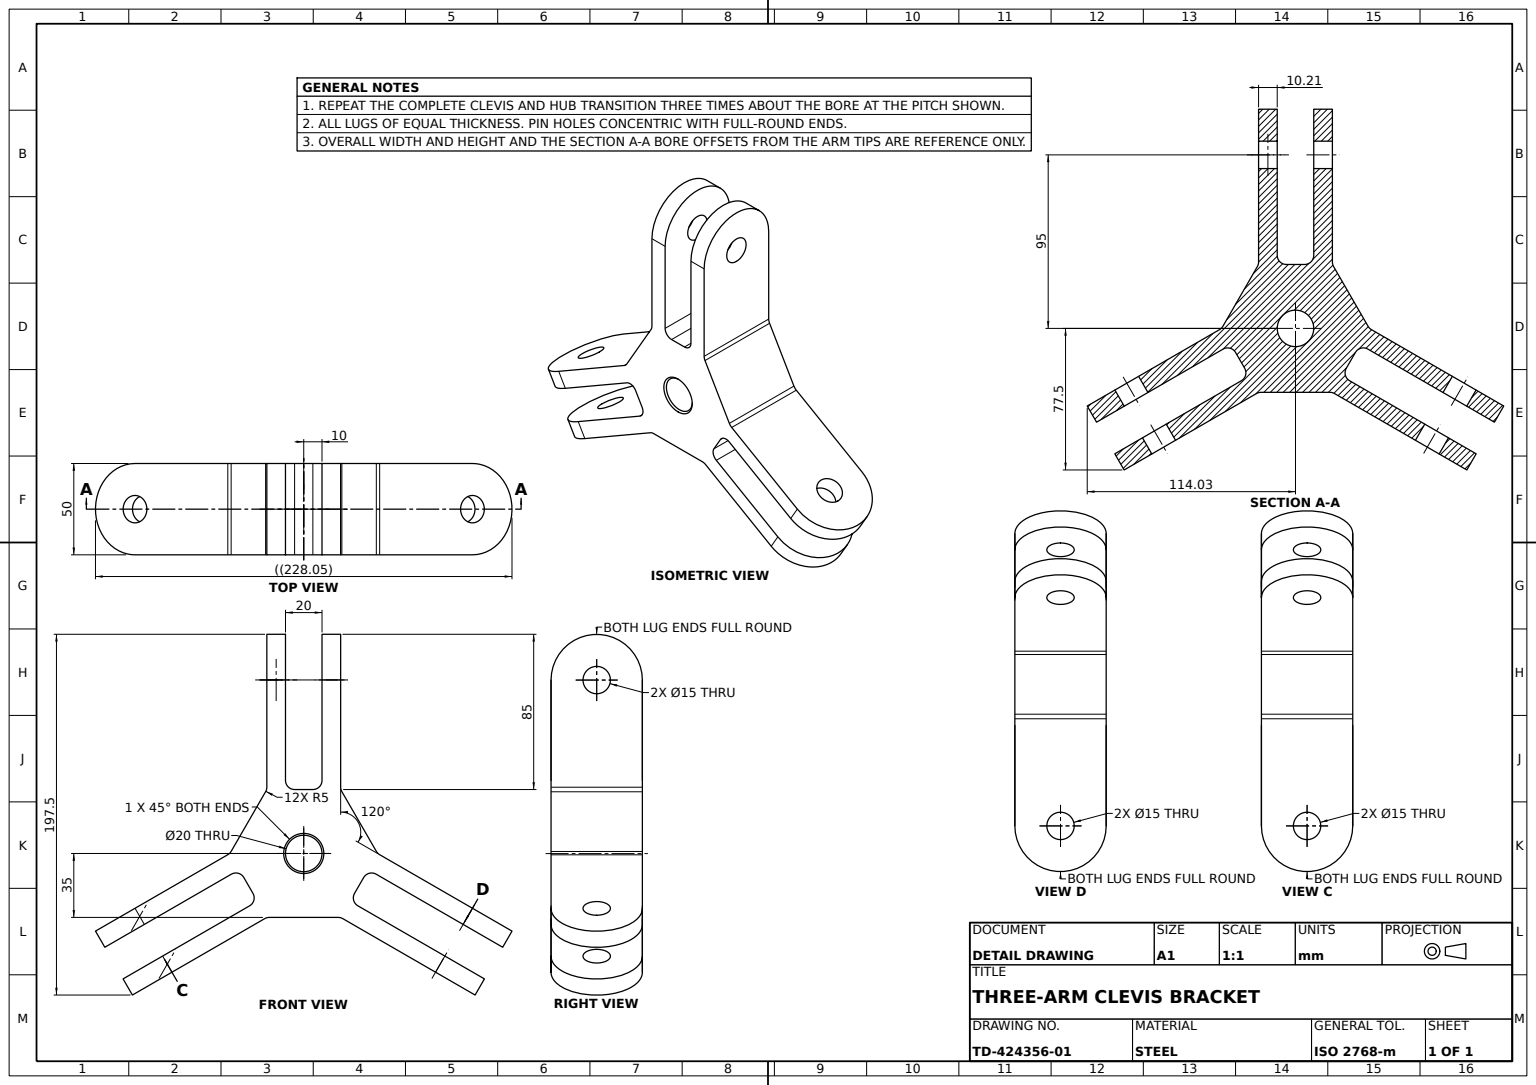
from build123d import *

# Parameters (mm, degrees)
THREE_ARM_BODY_50MM_DEPTH = 25
ARM_END_ROUND_B_RADIUS    = 25
ARM_END_ROUND_B_LENGTH    = 10.207259422
ARM_EDGE_FILLET_1_RADIUS  = 25
ARM_EDGE_FILLET_1_LENGTH  = 10.207259422
ARM_END_ROUND_A_RADIUS    = 25
ARM_END_ROUND_A_LENGTH    = 10.207259422
ARM_EDGE_FILLET_2_RADIUS  = 25
ARM_EDGE_FILLET_2_LENGTH  = 10.207259422
ARM_EDGE_FILLET_3_RADIUS  = 25
ARM_EDGE_FILLET_3_LENGTH  = 10.207259422
ARM_END_ROUND_C_RADIUS    = 25
ARM_END_ROUND_C_LENGTH    = 10.207259422
PIN_HOLE_A_15_REACH       = 188.921
PIN_HOLE_A_SKETCH_R       = 7.5
PIN_HOLE_B_15_REACH       = 188.921
PIN_HOLE_B_SKETCH_R       = 7.5
PIN_HOLE_C_15_REACH       = 183.779
PIN_HOLE_C_SKETCH_R       = 7.5
CENTER_BORE_SKETCH_R      = 10
CENTER_BORE_20_DEPTH      = 50
HUB_FILLET_R5_1_R         = 5
HUB_FILLET_R5_2_R         = 5
BORE_CHAMFER_1X45_SIZE    = 1


with BuildPart() as part:
    # Three-Arm Profile Sketch → Three-Arm Body 50mm (new, symmetric)
    with BuildSketch(Plane(origin=(0, 0, 0), x_dir=(1, 0, 0), z_dir=(0, 1, 0))):
        Polygon((-20.207259422, 35), (-20.207259422, 120), (-10, 120), (-10, 35), (10, 35), (10, 120), (20.207259422, 120), (20.207259422, 35), (40.414518843, 0), (114.026678165, -42.5), (108.923048454, -51.339745962), (35.310889132, -8.839745962), (25.310889132, -26.160254038), (98.923048454, -68.660254038), (93.819418743, -77.5), (20.207259422, -35), (-20.207259422, -35), (-93.819418743, -77.5), (-98.923048454, -68.660254038), (-25.310889132, -26.160254038), (-35.310889132, -8.839745962), (-108.923048454, -51.339745962), (-114.026678165, -42.5), (-40.414518843, 0), align=None)
    extrude(amount=THREE_ARM_BODY_50MM_DEPTH, both=True)

    # Arm End Round B: full round fillet: the end face becomes a half cylinder, R = half its width
    arm_end_round_b_face = Plane((-96.371233599, 0, 73.080127019), x_dir=(0.5, 0, 0.866025403784), z_dir=(-0.866025403784, 0, 0.5))  # on the end face: x along it, z out of the body
    arm_end_round_b_slab = arm_end_round_b_face.offset(-ARM_END_ROUND_B_RADIUS / 2) * Box(ARM_END_ROUND_B_LENGTH, 2 * ARM_END_ROUND_B_RADIUS, ARM_END_ROUND_B_RADIUS, mode=Mode.PRIVATE)  # the body's end, R deep
    arm_end_round_b_round = Plane((-74.720598504, 0, 60.580127019), x_dir=(-0.866025403784, 0, 0.5), z_dir=(0.5, 0, 0.866025403784)) * Cylinder(ARM_END_ROUND_B_RADIUS, ARM_END_ROUND_B_LENGTH, mode=Mode.PRIVATE)  # its axis R under the face
    add(arm_end_round_b_slab - arm_end_round_b_round, mode=Mode.SUBTRACT)

    # Arm Edge Fillet 1: full round fillet: the end face becomes a half cylinder, R = half its width
    arm_edge_fillet_1_face = Plane((-111.47486331, 0, 46.919872981), x_dir=(0.5, 0, 0.866025403784), z_dir=(-0.866025403784, 0, 0.5))  # on the end face: x along it, z out of the body
    arm_edge_fillet_1_slab = arm_edge_fillet_1_face.offset(-ARM_EDGE_FILLET_1_RADIUS / 2) * Box(ARM_EDGE_FILLET_1_LENGTH, 2 * ARM_EDGE_FILLET_1_RADIUS, ARM_EDGE_FILLET_1_RADIUS, mode=Mode.PRIVATE)  # the body's end, R deep
    arm_edge_fillet_1_round = Plane((-89.824228215, 0, 34.419872981), x_dir=(-0.866025403784, 0, 0.5), z_dir=(0.5, 0, 0.866025403784)) * Cylinder(ARM_EDGE_FILLET_1_RADIUS, ARM_EDGE_FILLET_1_LENGTH, mode=Mode.PRIVATE)  # its axis R under the face
    add(arm_edge_fillet_1_slab - arm_edge_fillet_1_round, mode=Mode.SUBTRACT)

    # Arm End Round A: full round fillet: the end face becomes a half cylinder, R = half its width
    arm_end_round_a_face = Plane((96.371233599, 0, 73.080127019), x_dir=(0.5, 0, -0.866025403784), z_dir=(0.866025403784, 0, 0.5))  # on the end face: x along it, z out of the body
    arm_end_round_a_slab = arm_end_round_a_face.offset(-ARM_END_ROUND_A_RADIUS / 2) * Box(ARM_END_ROUND_A_LENGTH, 2 * ARM_END_ROUND_A_RADIUS, ARM_END_ROUND_A_RADIUS, mode=Mode.PRIVATE)  # the body's end, R deep
    arm_end_round_a_round = Plane((74.720598504, 0, 60.580127019), x_dir=(0.866025403784, 0, 0.5), z_dir=(0.5, 0, -0.866025403784)) * Cylinder(ARM_END_ROUND_A_RADIUS, ARM_END_ROUND_A_LENGTH, mode=Mode.PRIVATE)  # its axis R under the face
    add(arm_end_round_a_slab - arm_end_round_a_round, mode=Mode.SUBTRACT)

    # Arm Edge Fillet 2: full round fillet: the end face becomes a half cylinder, R = half its width
    arm_edge_fillet_2_face = Plane((111.47486331, 0, 46.919872981), x_dir=(0.5, 0, -0.866025403784), z_dir=(0.866025403784, 0, 0.5))  # on the end face: x along it, z out of the body
    arm_edge_fillet_2_slab = arm_edge_fillet_2_face.offset(-ARM_EDGE_FILLET_2_RADIUS / 2) * Box(ARM_EDGE_FILLET_2_LENGTH, 2 * ARM_EDGE_FILLET_2_RADIUS, ARM_EDGE_FILLET_2_RADIUS, mode=Mode.PRIVATE)  # the body's end, R deep
    arm_edge_fillet_2_round = Plane((89.824228215, 0, 34.419872981), x_dir=(0.866025403784, 0, 0.5), z_dir=(0.5, 0, -0.866025403784)) * Cylinder(ARM_EDGE_FILLET_2_RADIUS, ARM_EDGE_FILLET_2_LENGTH, mode=Mode.PRIVATE)  # its axis R under the face
    add(arm_edge_fillet_2_slab - arm_edge_fillet_2_round, mode=Mode.SUBTRACT)

    # Arm Edge Fillet 3: full round fillet: the end face becomes a half cylinder, R = half its width
    arm_edge_fillet_3_face = Plane((15.103629711, 0, -120), x_dir=(-1, 0, 0), z_dir=(0, 0, -1))  # on the end face: x along it, z out of the body
    arm_edge_fillet_3_slab = arm_edge_fillet_3_face.offset(-ARM_EDGE_FILLET_3_RADIUS / 2) * Box(ARM_EDGE_FILLET_3_LENGTH, 2 * ARM_EDGE_FILLET_3_RADIUS, ARM_EDGE_FILLET_3_RADIUS, mode=Mode.PRIVATE)  # the body's end, R deep
    arm_edge_fillet_3_round = Plane((15.103629711, 0, -95), x_dir=(0, 0, -1), z_dir=(-1, 0, 0)) * Cylinder(ARM_EDGE_FILLET_3_RADIUS, ARM_EDGE_FILLET_3_LENGTH, mode=Mode.PRIVATE)  # its axis R under the face
    add(arm_edge_fillet_3_slab - arm_edge_fillet_3_round, mode=Mode.SUBTRACT)

    # Arm End Round C: full round fillet: the end face becomes a half cylinder, R = half its width
    arm_end_round_c_face = Plane((-15.103629711, 0, -120), x_dir=(1, 0, 0), z_dir=(0, 0, -1))  # on the end face: x along it, z out of the body
    arm_end_round_c_slab = arm_end_round_c_face.offset(-ARM_END_ROUND_C_RADIUS / 2) * Box(ARM_END_ROUND_C_LENGTH, 2 * ARM_END_ROUND_C_RADIUS, ARM_END_ROUND_C_RADIUS, mode=Mode.PRIVATE)  # the body's end, R deep
    arm_end_round_c_round = Plane((-15.103629711, 0, -95), x_dir=(0, 0, -1), z_dir=(1, 0, 0)) * Cylinder(ARM_END_ROUND_C_RADIUS, ARM_END_ROUND_C_LENGTH, mode=Mode.PRIVATE)  # its axis R under the face
    add(arm_end_round_c_slab - arm_end_round_c_round, mode=Mode.SUBTRACT)

    # Pin Hole A _15: up to this face of the body (flat: up to its plane)
    pin_hole_a_15_end = Plane(part.part.faces().sort_by_distance((75.066762447, 0, 20.006482173))[0])
    # Pin Hole A Sketch → Pin Hole A _15 (cut, up to the picked face)
    with BuildSketch(Plane(origin=(-10.103629711, 0, 17.5), x_dir=(0.8660254037844392, 0, 0.49999999999999917), z_dir=(-0.49999999999999917, 0, 0.8660254037844392)), mode=Mode.PRIVATE) as pin_hole_a_15_sk1:
        with Locations((95, 0)):
            Circle(PIN_HOLE_A_SKETCH_R)
    pin_hole_a_15_tool1 = split(extrude(pin_hole_a_15_sk1.sketch, amount=-PIN_HOLE_A_15_REACH, mode=Mode.PRIVATE), bisect_by=pin_hole_a_15_end, keep=Keep.BOTH, mode=Mode.PRIVATE)
    add(pin_hole_a_15_tool1.solids().sort_by(Axis((72.168784, 0, 65), (0.49999999999999917, 0, -0.8660254037844392)))[0], mode=Mode.SUBTRACT)

    # Pin Hole B _15: up to this face of the body (flat: up to its plane)
    pin_hole_b_15_end = Plane(part.part.faces().sort_by_distance((-75.066762447, 0, 20.006482173))[0])
    # Pin Hole B Sketch → Pin Hole B _15 (cut, up to the picked face)
    with BuildSketch(Plane(origin=(10.103629711, 0, 17.5), x_dir=(0.86602540378444, 0, -0.4999999999999976), z_dir=(0.4999999999999976, 0, 0.86602540378444)), mode=Mode.PRIVATE) as pin_hole_b_15_sk1:
        with Locations((-95, 0)):
            Circle(PIN_HOLE_B_SKETCH_R)
    pin_hole_b_15_tool1 = split(extrude(pin_hole_b_15_sk1.sketch, amount=-PIN_HOLE_B_15_REACH, mode=Mode.PRIVATE), bisect_by=pin_hole_b_15_end, keep=Keep.BOTH, mode=Mode.PRIVATE)
    add(pin_hole_b_15_tool1.solids().sort_by(Axis((-72.168784, 0, 65), (-0.4999999999999976, 0, -0.86602540378444)))[0], mode=Mode.SUBTRACT)

    # Pin Hole C _15: up to this face of the body (flat: up to its plane)
    pin_hole_c_15_end = Plane(part.part.faces().sort_by_distance((20.207259422, 0, -75.012964345))[0])
    # Pin Hole C Sketch → Pin Hole C _15 (cut, up to the picked face)
    with BuildSketch(Plane.ZY.offset(20.207259422), mode=Mode.PRIVATE) as pin_hole_c_15_sk1:
        with Locations((-95, 0)):
            Circle(PIN_HOLE_C_SKETCH_R)
    pin_hole_c_15_tool1 = split(extrude(pin_hole_c_15_sk1.sketch, amount=-PIN_HOLE_C_15_REACH, mode=Mode.PRIVATE), bisect_by=pin_hole_c_15_end, keep=Keep.BOTH, mode=Mode.PRIVATE)
    add(pin_hole_c_15_tool1.solids().sort_by(Axis((-20.207259, 0, -95), (1, 0, 0)))[0], mode=Mode.SUBTRACT)

    # Center Bore Sketch → Center Bore _20 (cut)
    with BuildSketch(Plane.XZ.offset(25)):
        with Locations(Location((0, 0, 0), (0, 0, 270))):
            Circle(CENTER_BORE_SKETCH_R)
    extrude(amount=-CENTER_BORE_20_DEPTH, mode=Mode.SUBTRACT)

    # Hub Fillet R5 1
    hub_fillet_r5_1_edges = [part.edges().sort_by_distance(p)[0] for p in [
        (35.310889132, 0, 8.839745962),
        (25.310889132, 0, 26.160254038),
        (-25.310889132, 0, 26.160254038),
        (-35.310889132, 0, 8.839745962),
        (-10, 0, -35),
        (10, 0, -35),
    ]]
    fillet(hub_fillet_r5_1_edges, radius=HUB_FILLET_R5_1_R)

    # Hub Fillet R5 2
    hub_fillet_r5_2_edges = [part.edges().sort_by_distance(p)[0] for p in [
        (20.207259422, 0, -35),
        (40.414518843, 0, 0),
        (20.207259422, 0, 35),
        (-20.207259422, 0, 35),
        (-40.414518843, 0, 0),
        (-20.207259422, 0, -35),
    ]]
    fillet(hub_fillet_r5_2_edges, radius=HUB_FILLET_R5_2_R)

    # Bore Chamfer 1x45
    bore_chamfer_1x45_edges = [part.edges().sort_by_distance(p)[0] for p in [
        (0, -25, 10),
        (0, 25, 10),
    ]]
    chamfer(bore_chamfer_1x45_edges, length=BORE_CHAMFER_1X45_SIZE)


solid = part.part
